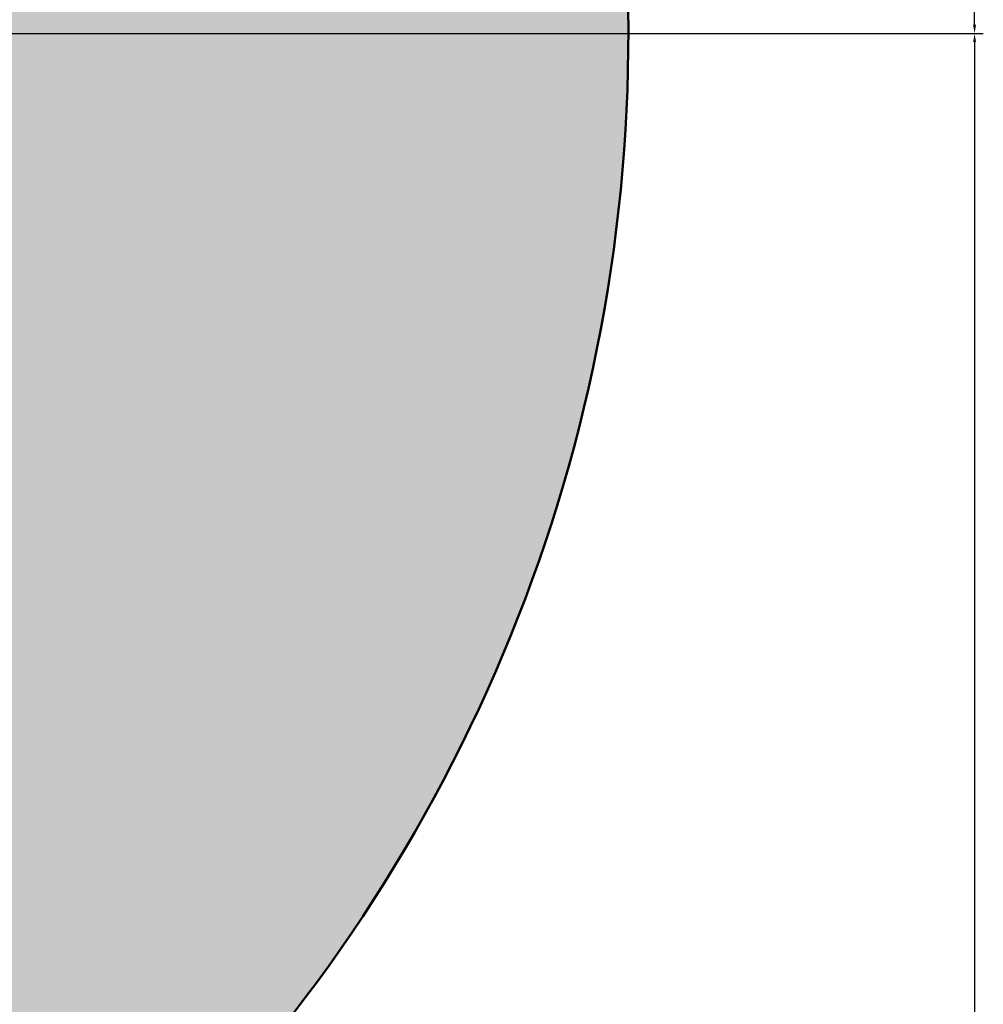
# Model space of a CAD drawing. Units: inches. Extents: x -13 to 107, y -48 to 102.
# Tile 7 of 13: x 48 to 68, y -7 to 14. Entities that reach past the tile are written whole.
import ezdxf

# ---------------------------------------------------------------- set-up
doc = ezdxf.new("R2010")
doc.units = ezdxf.units.IN
doc.header["$MEASUREMENT"] = 0
for name, color, linetype, lineweight in [('M-DIMS', 2, 'Continuous', 18), ('M-HATC', 8, 'Continuous', 18), ('M-OUTL', 7, 'Continuous', 50)]:
    doc.layers.add(name, color=color, linetype=linetype, lineweight=lineweight)
doc.styles.get("Standard").update_dxf_attribs({"font": 'arial.ttf'})
doc.dimstyles.get("Standard").update_dxf_attribs({"dimtxt": 0.18, "dimasz": 0.18, "dimexe": 0.18, "dimexo": 0.0625, "dimgap": 0.09, "dimtad": 0, "dimtih": 1, "dimtoh": 1, "dimdec": 4, "dimzin": 0, "dimdsep": 46, "dimtxsty": 'Standard', "dimcen": 0.09, "dimadec": 0, "dimazin": 0, "dimtfac": 1, "dimtdec": 4, "dimtofl": 0, "dimtmove": 0, "dimatfit": 3, "dimfxl": 1, "dimtolj": 1, "dimtzin": 0, "dimarcsym": 0})

# ---------------------------------------------------------------- blocks, each defined once
blk = doc.blocks.new('*D3')
at = {"layer": 'Defpoints', "color": 0, "transparency": 16777216}
for p in [(27.547, 13.408), (67.679, 13.408), (27.547, -36.592)]:
    blk.add_point(p, dxfattribs=at)
at = {"layer": 'M-DIMS', "color": 0, "lineweight": -2, "transparency": 16777216}
for p, q in [((27.609, 13.408), (67.859, 13.408)), ((67.679, 13.228), (67.679, -11.41)), ((67.679, -36.412), (67.679, -11.774)), ((27.609, -36.592), (67.859, -36.592))]:
    blk.add_line(p, q, dxfattribs=at)
at = {"layer": 'M-DIMS', "color": 0, "transparency": 16777216}
for points in [[(67.649, 13.228), (67.709, 13.228), (67.679, 13.408)], [(67.649, -36.412), (67.709, -36.412), (67.679, -36.592)]]:
    blk.add_solid(points, dxfattribs=at)
at = {"layer": 'M-DIMS', "color": 0, "transparency": 16777216, "insert": (67.679, -11.592), "char_height": 0.18, "attachment_point": 5}
blk.add_mtext('\\A1;50', dxfattribs=at)
blk = doc.blocks.new('*D4')
at = {"layer": 'Defpoints', "color": 0, "transparency": 16777216}
for p in [(27.547, 78.408), (67.679, 78.408), (27.547, 13.408)]:
    blk.add_point(p, dxfattribs=at)
at = {"layer": 'M-DIMS', "color": 0, "lineweight": -2, "transparency": 16777216}
for p, q in [((27.609, 78.408), (67.859, 78.408)), ((67.679, 78.228), (67.679, 46.09)), ((67.679, 13.588), (67.679, 45.726)), ((27.609, 13.408), (67.859, 13.408))]:
    blk.add_line(p, q, dxfattribs=at)
at = {"layer": 'M-DIMS', "color": 0, "transparency": 16777216}
for points in [[(67.649, 78.228), (67.709, 78.228), (67.679, 78.408)], [(67.649, 13.588), (67.709, 13.588), (67.679, 13.408)]]:
    blk.add_solid(points, dxfattribs=at)
at = {"layer": 'M-DIMS', "color": 0, "transparency": 16777216, "insert": (67.679, 45.908), "char_height": 0.18, "attachment_point": 5}
blk.add_mtext('\\A1;65', dxfattribs=at)
blk = doc.blocks.new('*D8')
at = {"layer": 'Defpoints', "color": 0, "transparency": 16777216}
for p in [(27.547, 13.408), (50.882, -9.927)]:
    blk.add_point(p, dxfattribs=at)
at = {"layer": 'M-DIMS', "color": 0, "lineweight": -2, "transparency": 16777216}
for p, q in [((27.457, 13.408), (27.637, 13.408)), ((27.547, 13.318), (27.547, 13.498)), ((64.882, -23.927), (51.009, -10.054)), ((65.062, -23.927), (64.882, -23.927))]:
    blk.add_line(p, q, dxfattribs=at)
at = {"layer": 'M-DIMS', "color": 0, "transparency": 16777216}
blk.add_solid([(51.03, -10.033), (50.988, -10.075), (50.882, -9.927)], dxfattribs=at)
at = {"layer": 'M-DIMS', "color": 0, "transparency": 16777216, "insert": (65.562, -23.927), "char_height": 0.18, "attachment_point": 5}
blk.add_mtext('\\A1;2X R33', dxfattribs=at)

msp = doc.modelspace()

# ---------------------------------------------------------------- hatches: boundary and pattern name
at = {"layer": 'M-HATC'}
h = msp.add_hatch(color=256, dxfattribs=at)
h.set_gradient(color1=(88, 186, 72), color2=(241, 235, 31), tint=1)
h.paths.add_polyline_path([(45.86, -14.044, 0.420873), (54.577, 32.339, -0.184081), (43.437, 76.537, 1.124637), (11.657, 76.537, -0.184081), (0.517, 32.339, 0.420873), (9.234, -14.044, -0.304084), (17.743, -34.622, 1.220926), (37.351, -34.622, -0.304084)])
h.paths.add_polyline_path([(33.479, -5.692, 0.859727), (21.615, -5.692, -0.111692), (13.972, -1.28, 0.859727), (8.04, 8.995, -0.111692), (8.04, 17.82, 0.859727), (13.972, 28.095, -0.111692), (21.615, 32.508, 0.859727), (33.479, 32.508, -0.111692), (41.122, 28.095, 0.859727), (47.054, 17.82, -0.111692), (47.054, 8.995, 0.859727), (41.122, -1.28, -0.111692)], flags=16)
h.paths.add_polyline_path([(32.547, -36.592, -1), (22.547, -36.592, -1)], flags=16)
h.paths.add_polyline_path([(17.547, 78.408, -1), (37.547, 78.408, -1)], flags=16)

# ---------------------------------------------------------------- linework, layer by layer
at = {"layer": 'M-OUTL'}
msp.add_arc((27.547, 13.408), 33, 303.707, 35.0067, dxfattribs=at)

# ---------------------------------------------------------------- dimensions: what is measured, and where the dimension line sits
at = {"layer": 'M-DIMS'}
for base, p1, p2, picture, middle in [((67.679, 78.408), (27.547, 13.408), (27.547, 78.408), '*D4', (67.679, 45.908)), ((67.679, 13.408), (27.547, -36.592), (27.547, 13.408), '*D3', (67.679, -11.592))]:
    dim = msp.add_linear_dim(base=base, p1=p1, p2=p2, angle=90, dimstyle='Standard', override={"dimdec": 0, "dimlfac": 1, "dimrnd": 0, "dimzin": 0, "dimdsep": 46, "dimlunit": 2}, dxfattribs=at)
    dim.commit()
    dim.dimension.update_dxf_attribs({"geometry": picture, "text_midpoint": middle})
dim = msp.add_radius_dim(center=(27.547, 13.408), mpoint=(50.882, -9.927), text='2X <>', dimstyle='Standard', override={"dimdec": 0, "dimlfac": 1, "dimrnd": 0, "dimzin": 0, "dimdsep": 46, "dimlunit": 2}, dxfattribs=at)
dim.commit()
dim.dimension.update_dxf_attribs({"geometry": '*D8', "text_midpoint": (65.562, -23.927), "dimtype": 164})

doc.saveas('drawing.dxf')
